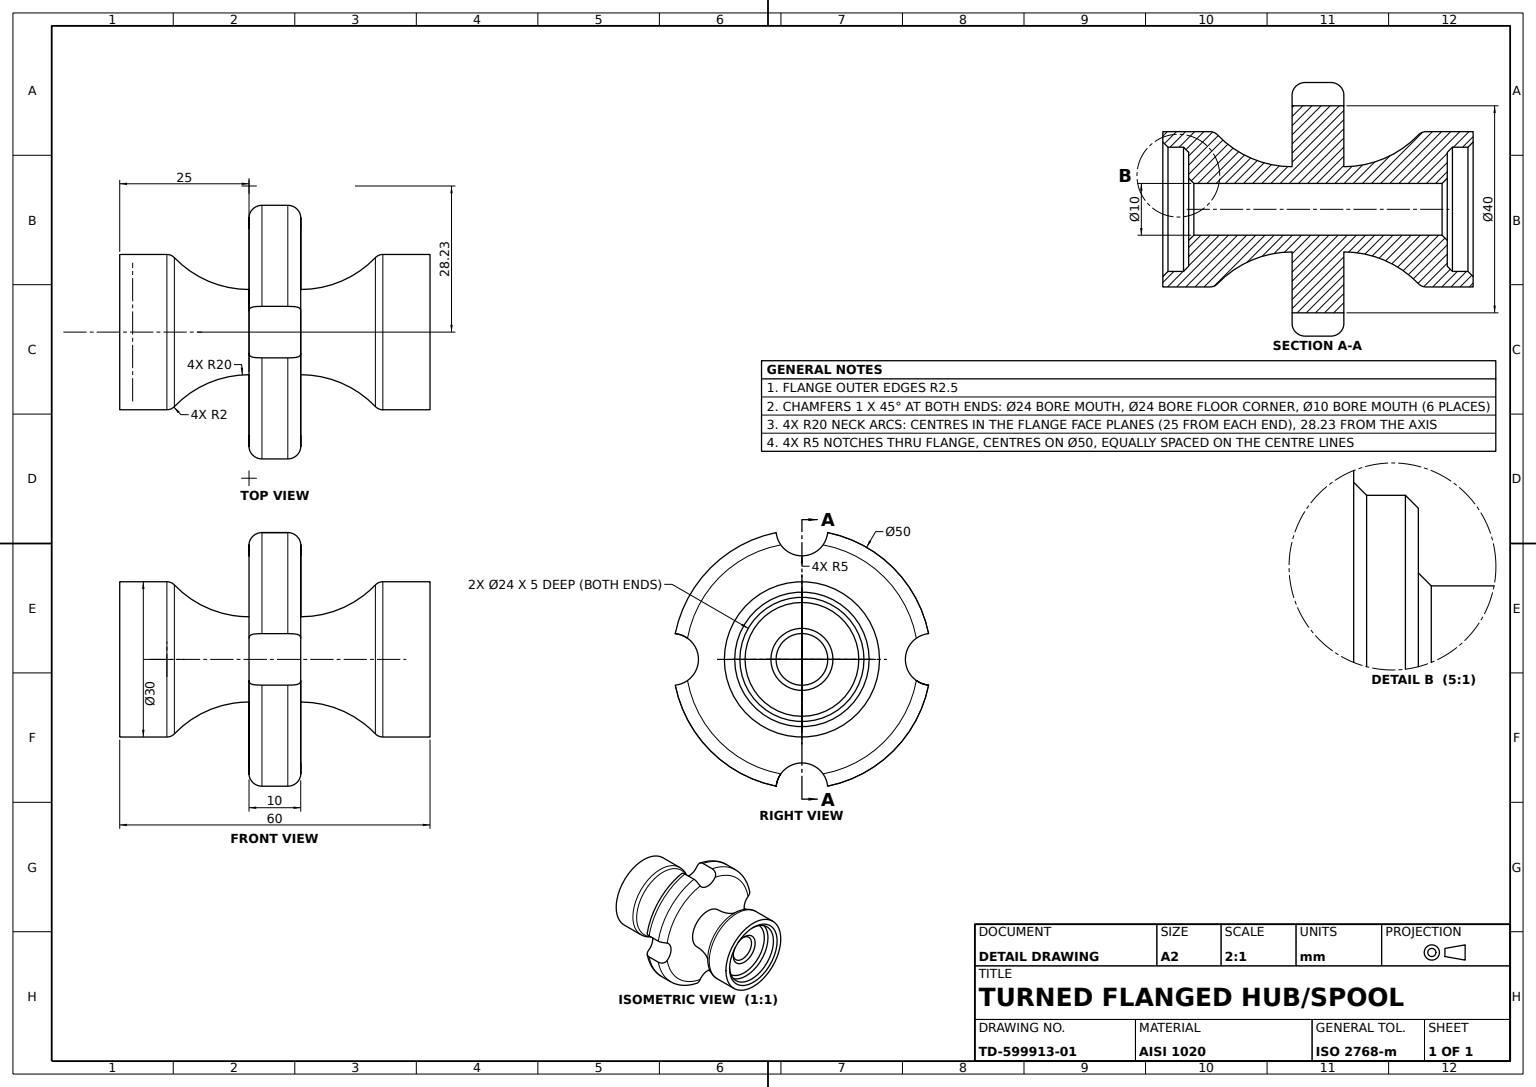
SolidWorks part; units mm, degrees
material "AISI 1020"
ref_plane "Front Plane" through (0, 0, 0) normal (0, 0, 1) x (1, 0, 0)
ref_plane "Top Plane" through (0, 0, 0) normal (0, 1, 0) x (1, 0, 0)
ref_plane "Right Plane" through (0, 0, 0) normal (1, 0, 0) x (0, 0, -1)
sketch "Hub Profile Sketch" plane through (0, 0, 0) normal (0, 0, 1) x (1, 0, 0)
  line L0 (0, 60) -> (0, 0) construction
  line L1 (-44.229, 30) -> (41.4446, 30) construction
  line L2 (12, 0) -> (12, 5)
  line L3 (12, 5) -> (5, 5)
  line L4 (5, 5) -> (5, 55)
  line L5 (5, 55) -> (12, 55)
  line L6 (12, 55) -> (12, 60)
  line L7 (12, 60) -> (15, 60)
  line L8 (15, 60) -> (15, 50)
  line L9 (8.2288, 35) -> (25, 35)
  line L10 (25, 35) -> (25, 25)
  line L11 (8.2288, 25) -> (25, 25)
  line L12 (15, 0) -> (15, 10)
  line L13 (12, 0) -> (15, 0)
  arc A0 (15, 50) -> (8.2288, 35) centre (28.2288, 35) ccw
  arc A1 (15, 10) -> (8.2288, 25) centre (28.2288, 25) cw
  point P23 (25, 30)
  dimension "D3" = 20
  dimension "D1" = 60
  dimension "D4" = 12
  dimension "D5" = 5
  dimension "D6" = 5
  dimension "D7" = 5
  dimension "D8" = 10
  dimension "D9" = 15
  dimension "D10" = 5
  dimension "D11" = 25
revolve "Hub Body Revolve" add sketch "Hub Profile Sketch" angle 360 about L0
fillet "Flange Fillet R2.5" radius 2.5 2 edges at (0, 25, 25) (0, 35, 25)
sketch "Flange Notch Sketch" plane through (0, 35, 0) normal (0, 1, 0) x (1, 0, 0)
  line L0 (0, 31.6822) -> (0, -30.3342) construction
  circle A0 centre (0, 0) radius 25 construction
  circle A1 centre (0, 0) radius 25 construction
  circle A2 centre (0, 25) radius 5
  circle A3 centre (25, 0) radius 5
  circle A4 centre (0, -25) radius 5
  circle A5 centre (-25, 0) radius 5
  point P17 (0, 0)
  dimension "D1" = 10
  dimension "D2" = 4
extrude "Flange Notches 4x" cut sketch "Flange Notch Sketch" against normal up to next
chamfer "Edge Chamfer 1x45 A" distance 1 angle 45 4 edges at (0, 0, 12) (0, 5, 5) (0, 55, 5) (0, 60, 12)
fillet "Edge Fillet R2" radius 2 2 edges at (0, 50, 15) (0, 10, 15)
chamfer "Edge Chamfer 1x45 B" distance 1 angle 45 2 edges at (0, 55, 12) (0, 5, 12)
